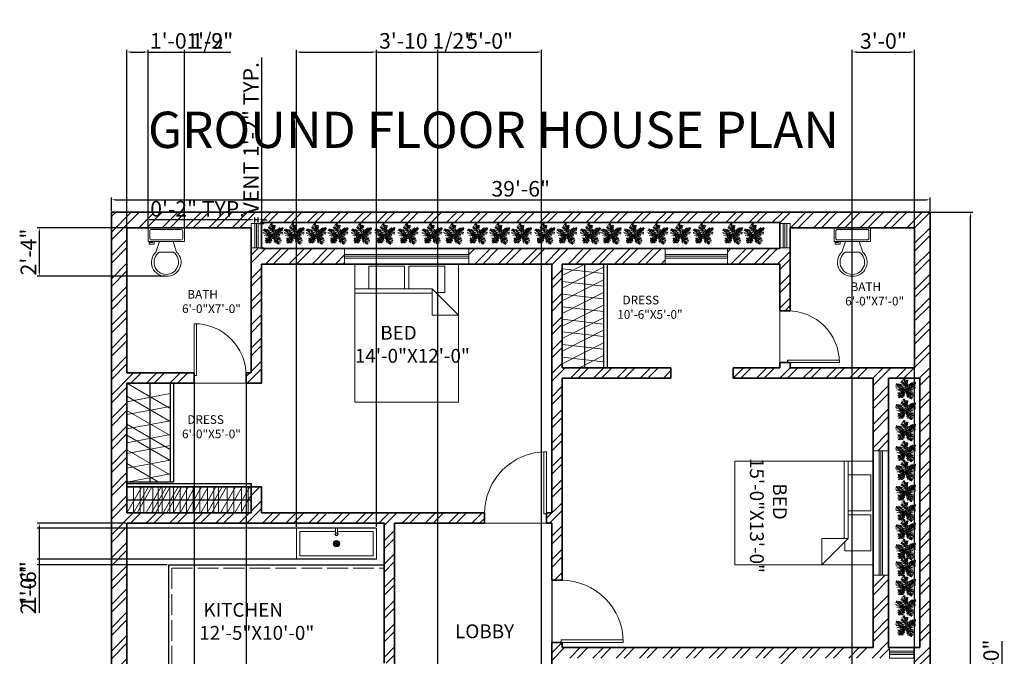
# Model space of a CAD drawing. Units: inches. Extents: x 177 to 1423, y 532 to 2503.
# Tile 4 of 5: x 197 to 768, y 1096 to 1465. Entities that reach past the tile are written whole.
import ezdxf

# ---------------------------------------------------------------- set-up
doc = ezdxf.new("R2010")
doc.units = ezdxf.units.IN
doc.linetypes.add('ACAD_ISO02W100', pattern=[15, 12, -3])
for name, color, linetype, lineweight in [('A-ANNO-DIMS', 2, 'Continuous', 18), ('A-ANNO-TITL', 7, 'Continuous', 35), ('A-AREA-IDEN', 7, 'Continuous', 18), ('A-DOOR', 4, 'Continuous', 18), ('A-FLOR-CASE', 8, 'Continuous', 25), ('A-FLOR-CASE-HIDN', 8, 'ACAD_ISO02W100', 13), ('A-FLOR-CASE-PATT', 252, 'Continuous', 13), ('A-FLOR-FIXT', 9, 'Continuous', 18), ('A-FURN', 8, 'Continuous', 18), ('A-GLAZ', 244, 'Continuous', 18), ('A-WALL', 7, 'Continuous', 35), ('A-WALL-PATT', 252, 'Continuous', 13), ('L-PLNT', 94, 'Continuous', 13)]:
    doc.layers.add(name, color=color, linetype=linetype, lineweight=lineweight)
doc.styles.get("Standard").update_dxf_attribs({"font": 'arial.ttf'})
doc.dimstyles.new('ISO-25', dxfattribs={"dimtxt": 9, "dimasz": 2.5, "dimexe": 1.25, "dimexo": 0.625, "dimtad": 1, "dimlunit": 3, "dimtxsty": 'Standard', "dimcen": 2.5, "dimadec": 0, "dimazin": 0, "dimtfac": 1, "dimtmove": 0, "dimatfit": 3, "dimfxl": 1, "dimarcsym": 0})

# ---------------------------------------------------------------- blocks, each defined once
blk = doc.blocks.new('*U2')
for p, q in [((0, 0), (0, -6)), ((40, 0), (40, -6))]:
    blk.add_line(p, q)
blk.add_lwpolyline([(0, 0), (0, 40), (1.75, 40), (1.75, 0)], close=True)
blk.add_arc((0, 0), 40, 0, 90)
blk = doc.blocks.new('*U3')
for p, q in [((0, 0), (0, -6)), ((-40, 0), (-40, -6))]:
    blk.add_line(p, q)
blk.add_lwpolyline([(0, 0), (0, 40), (-1.75, 40), (-1.75, 0)], close=True)
blk.add_arc((0, 0), 40, 90, 180)
blk = doc.blocks.new('Bed - Queen')
for p, q in [((0, -80.00003), (0, 0)), ((0, 0), (59.99999, 0)), ((59.99999, 0), (59.99999, -80.00003)), ((7.99999, -1.2), (28.79998, -1.2)), ((7.99999, -14.4), (7.99999, -1.2)), ((28.79998, -1.2), (28.79998, -14.4)), ((31.19999, -1.2), (51.99999, -1.2)), ((31.19999, -14.4), (31.19999, -1.2)), ((51.99999, -1.2), (51.99999, -16.4)), ((0, -14.4), (44.8, -14.4)), ((44.8, -16.8), (0, -16.8)), ((59.99999, -29.6), (44.8, -14.4)), ((44.8, -14.4), (44.8, -29.6)), ((51.99999, -16.4), (46.79936, -16.4)), ((44.8, -29.6), (59.99999, -29.6)), ((59.99999, -80.00003), (0, -80.00003))]:
    blk.add_line(p, q)
blk = doc.blocks.new('*U12')
for p, q in [((9.5, -6), (9.5, -2)), ((-10, -8.5), (-8, -8.5)), ((-10, -9.5), (-10, -8.5)), ((-7, -9.5), (-10, -9.5)), ((-8, -8.5), (-8, -8)), ((-7, -8), (-7, -9.5)), ((-4, -8), (-6, -14)), ((4, -8), (6, -14)), ((4, -14), (-4, -14))]:
    blk.add_line(p, q)
blk.add_lwpolyline([(10.5, -8), (10.5, 0), (-10.5, 0), (-10.5, -8)], close=True)
for points in [[(-9.5, -2), (-9.5, -6)], [(8.5, -1), (-8.5, -1)], [(-8.5, -7), (8.5, -7)]]:
    blk.add_lwpolyline(points)
for centre, radius, start, end in [((-8.625, -1.875), 0.8839, 81.8699, 188.1301), ((8.625, -1.875), 0.8839, 351.8699, 98.1301), ((-8.625, -6.125), 0.8839, 171.869898, 278.1301), ((8.625, -6.125), 0.8839, 261.8699, 8.1301), ((-0.4772, -19.9188), 8.0953, 133.01722, 273.38), ((0.0374, -19.8731), 7.127, 124.50543, 269.7), ((-0.0373, -19.8731), 7.127, 270.3, 55.4946), ((0.4773, -19.9188), 8.0953, 266.62, 46.9828)]:
    blk.add_arc(centre, radius, start, end)
blk = doc.blocks.new('*U9')
for p, q in [((9.5, -6), (9.5, -2)), ((-10, -8.5), (-8, -8.5)), ((-10, -9.5), (-10, -8.5)), ((-7, -9.5), (-10, -9.5)), ((-8, -8.5), (-8, -8)), ((-7, -8), (-7, -9.5)), ((-4, -8), (-6, -14)), ((4, -8), (6, -14)), ((4, -14), (-4, -14))]:
    blk.add_line(p, q)
blk.add_lwpolyline([(10.5, -8), (10.5, 0), (-10.5, 0), (-10.5, -8)], close=True)
for points in [[(-9.5, -2), (-9.5, -6)], [(8.5, -1), (-8.5, -1)], [(-8.5, -7), (8.5, -7)]]:
    blk.add_lwpolyline(points)
for centre, radius, start, end in [((-8.625, -1.875), 0.8839, 81.8699, 188.1301), ((8.625, -1.875), 0.8839, 351.8699, 98.1301), ((-8.625, -6.125), 0.8839, 171.869898, 278.1301), ((8.625, -6.125), 0.8839, 261.8699, 8.1301), ((-0.4772, -19.9188), 8.0953, 133.01722, 273.38), ((0.0374, -19.8731), 7.127, 124.50543, 269.7), ((-0.0373, -19.8731), 7.127, 270.3, 55.4946), ((0.4773, -19.9188), 8.0953, 266.62, 46.9828)]:
    blk.add_arc(centre, radius, start, end)
blk = doc.blocks.new('*U11')
for p, q in [((-8.737, 47.138), (-17.069, 52.711)), ((-10.186, 53.64), (-13.084, 55.962)), ((0, 0), (-10.5, 57)), ((-9.099, 51.782), (-6.563, 55.962)), ((-47.498, 19.737), (-55.83, 18.344)), ((-40.615, 13.7), (-55.105, 10.913)), ((-31.5, 4.5), (-52.5, 25.5)), ((-33.37, 6.269), (-52.207, 5.34)), ((-48.585, 21.131), (-49.309, 29.026)), ((-28.299, 3.483), (-47.86, -5.805)), ((-43.513, 28.561), (-42.427, 15.558)), ((-38.442, 26.239), (-34.819, 7.663)), ((-21.416, 3.018), (-38.079, -8.128)), ((-35.544, 28.097), (-24.314, 3.947)), ((0, 0), (-31.5, 4.5)), ((-14.533, 2.09), (-30.834, 25.31)), ((-15.982, 2.09), (-30.11, -9.521)), ((-3.665, 19.273), (-27.574, 35.527)), ((-5.114, 28.097), (-24.676, 40.636)), ((-24.314, 23.917), (-2.941, 13.7)), ((0, 0), (-22.5, -19.5)), ((-7.288, 39.707), (-21.778, 46.673)), ((-6.563, 1.161), (-21.416, -8.128)), ((-20.691, 13.7), (-1.129, 4.876)), ((-7.65, 43.423), (-2.578, 49.46)), ((-5.839, 35.992), (4.667, 48.067)), ((-5.114, 27.632), (10.463, 46.673)), ((-2.941, 16.486), (8.652, 37.85)), ((-1.129, 6.734), (9.014, 26.704)), ((0, 0), (27, 9)), ((0, 0), (18, -22.5)), ((3.942, 1.625), (11.187, 24.381)), ((6.478, 1.625), (26.04, -8.592)), ((10.101, 3.483), (17.708, 26.239)), ((11.187, 3.483), (30.749, -5.805)), ((16.259, 5.805), (23.142, 31.348)), ((18.07, 5.805), (35.096, -3.483)), ((22.055, 7.198), (27.489, 32.277)), ((24.229, 7.663), (46.688, 1.625)), ((27, 9), (48, 36)), ((27.127, 9.056), (31.112, 35.992)), ((29.662, 12.307), (48.137, 6.269)), ((31.836, 30.883), (32.561, 16.486)), ((33.285, 16.486), (48.862, 10.913)), ((35.096, 32.741), (37.27, 22.524)), ((36.183, 19.737), (48.137, 17.88)), ((38.719, 34.134), (41.979, 28.561)), ((40.53, 25.775), (48.862, 24.846)), ((43.791, 29.954), (51.036, 30.883)), ((44.153, 36.456), (45.239, 32.741)), ((-17.431, -15.094), (-42.789, -18.809)), ((-28.299, -29.026), (-42.789, -31.348)), ((-24.314, -21.596), (-42.427, -22.06)), ((-30.834, -34.135), (-42.427, -35.528)), ((-34.457, -39.708), (-40.978, -42.494)), ((-26.849, -26.24), (-40.253, -25.775)), ((-22.5, -19.5), (-37.5, -45)), ((-32.646, -36.921), (-31.921, -44.352)), ((-15.257, -12.772), (-30.11, -12.772)), ((-29.023, -30.884), (-27.936, -43.887)), ((-25.038, -23.918), (-22.865, -45.281)), ((-20.691, -18.345), (-17.793, -44.352)), ((-6.563, -5.805), (-19.967, -9.985)), ((-17.069, -15.094), (-12.721, -40.172)), ((-13.446, -11.378), (-8.737, -32.741)), ((-9.461, -8.592), (-6.201, -23.453)), ((-4.752, -3.483), (-3.665, -14.629)), ((2.493, -3.019), (-1.491, -20.202)), ((1.769, -2.555), (24.229, -9.521)), ((5.029, -6.27), (2.131, -25.775)), ((9.014, -11.378), (3.58, -35.992)), ((14.085, -16.951), (6.478, -40.172)), ((7.565, -9.056), (32.198, -14.629)), ((18.07, -22.524), (8.289, -45.745)), ((12.274, -15.094), (36.907, -18.809)), ((20.244, -30.419), (15.897, -44.816)), ((16.259, -19.738), (36.183, -22.989)), ((18, -22.5), (27, -52.5)), ((18.433, -22.524), (40.53, -29.026)), ((19.157, -25.311), (38.719, -33.206)), ((22.78, -37.85), (19.519, -48.532)), ((21.331, -32.741), (39.081, -40.636)), ((22.78, -38.314), (34.372, -44.816)), ((24.591, -45.745), (23.142, -50.854)), ((24.591, -43.423), (30.749, -47.603)), ((26.764, -49.925), (28.213, -50.854))]:
    blk.add_line(p, q)
blk = doc.blocks.new('*D15')
at = {"layer": 'A-ANNO-DIMS', "color": 0, "lineweight": -2, "transparency": 16777216}
for p, q in [((250.55, 1353.78), (250.55, 1361.61)), ((253.05, 1360.36), (722.05, 1360.36)), ((724.55, 1353.78), (724.55, 1361.61))]:
    blk.add_line(p, q, dxfattribs=at)
at = {"layer": 'A-ANNO-DIMS', "color": 0, "transparency": 16777216}
for points in [[(253.05, 1360.77), (253.05, 1359.94), (250.55, 1360.36)], [(722.05, 1360.77), (722.05, 1359.94), (724.55, 1360.36)]]:
    blk.add_solid(points, dxfattribs=at)
at = {"layer": 'Defpoints', "color": 0, "transparency": 16777216}
for p in [(724.55, 1360.36), (250.55, 1353.15), (724.55, 1353.15)]:
    blk.add_point(p, dxfattribs=at)
at = {"layer": 'A-ANNO-DIMS', "color": 0, "transparency": 16777216, "insert": (487.55, 1365.58), "char_height": 9, "attachment_point": 5}
blk.add_mtext('39\'-6"', dxfattribs=at)
blk = doc.blocks.new('*D16')
at = {"layer": 'A-ANNO-DIMS', "color": 0, "lineweight": -2, "transparency": 16777216}
for p, q in [((725.18, 1353.15), (749.29, 1353.15)), ((748.04, 638.65), (748.04, 1350.65)), ((725.18, 636.15), (749.29, 636.15))]:
    blk.add_line(p, q, dxfattribs=at)
at = {"layer": 'A-ANNO-DIMS', "color": 0, "transparency": 16777216}
for points in [[(747.63, 1350.65), (748.46, 1350.65), (748.04, 1353.15)], [(747.63, 638.65), (748.46, 638.65), (748.04, 636.15)]]:
    blk.add_solid(points, dxfattribs=at)
at = {"layer": 'Defpoints', "color": 0, "transparency": 16777216}
for p in [(724.55, 1353.15), (748.04, 1353.15), (724.55, 636.15)]:
    blk.add_point(p, dxfattribs=at)
at = {"layer": 'A-ANNO-DIMS', "color": 0, "transparency": 16777216, "insert": (742.82, 994.65), "char_height": 9, "attachment_point": 5, "rotation": 90}
blk.add_mtext('59\'-9"', dxfattribs=at)
blk = doc.blocks.new('WIN-GLAZING-72IN')
for p, q in [((72, 2), (0, 2)), ((72, 1), (0, 1)), ((72, 0), (0, 0))]:
    blk.add_line(p, q)
blk = doc.blocks.new('VENT-GLAZING-SHORT')
for p, q in [((14.07, 2), (0, 2)), ((14.07, 1), (0, 1)), ((14.07, 0), (0, 0))]:
    blk.add_line(p, q)
blk = doc.blocks.new('*D26')
at = {"layer": 'A-ANNO-DIMS', "color": 0, "lineweight": -2, "transparency": 16777216}
for p, q in [((337.66, 1346.69), (337.66, 1442.79)), ((336.18, 1346.69), (338.91, 1346.69)), ((337.66, 1335.12), (337.66, 1344.19)), ((336.18, 1332.62), (338.91, 1332.62))]:
    blk.add_line(p, q, dxfattribs=at)
at = {"layer": 'A-ANNO-DIMS', "color": 0, "transparency": 16777216}
for points in [[(337.25, 1344.19), (338.08, 1344.19), (337.66, 1346.69)], [(337.25, 1335.12), (338.08, 1335.12), (337.66, 1332.62)]]:
    blk.add_solid(points, dxfattribs=at)
at = {"layer": 'Defpoints', "color": 0, "transparency": 16777216}
for p in [(335.55, 1346.69), (337.66, 1346.69), (335.55, 1332.62)]:
    blk.add_point(p, dxfattribs=at)
at = {"layer": 'A-ANNO-DIMS', "color": 0, "transparency": 16777216, "insert": (332.52, 1395.99), "char_height": 9, "attachment_point": 5, "rotation": 90}
blk.add_mtext('VENT 1\'-2" TYP.', dxfattribs=at)
blk = doc.blocks.new('*D27')
at = {"layer": 'A-ANNO-DIMS', "color": 0, "lineweight": -2, "transparency": 16777216}
for p, q in [((331.05, 1348.8), (272.44, 1348.8)), ((333.55, 1347.32), (333.55, 1350.05)), ((335.55, 1348.8), (333.55, 1348.8)), ((335.55, 1347.32), (335.55, 1350.05)), ((338.05, 1348.8), (340.55, 1348.8))]:
    blk.add_line(p, q, dxfattribs=at)
at = {"layer": 'A-ANNO-DIMS', "color": 0, "transparency": 16777216}
for points in [[(331.05, 1349.22), (331.05, 1348.39), (333.55, 1348.8)], [(338.05, 1349.22), (338.05, 1348.39), (335.55, 1348.8)]]:
    blk.add_solid(points, dxfattribs=at)
at = {"layer": 'Defpoints', "color": 0, "transparency": 16777216}
for p in [(333.55, 1348.8), (333.55, 1346.69), (335.55, 1346.69)]:
    blk.add_point(p, dxfattribs=at)
at = {"layer": 'A-ANNO-DIMS', "color": 0, "transparency": 16777216, "insert": (300.5, 1354.02), "char_height": 9, "attachment_point": 5}
blk.add_mtext('0\'-2" TYP.', dxfattribs=at)
blk = doc.blocks.new('*D38')
at = {"layer": 'A-ANNO-DIMS', "color": 0, "lineweight": -2, "transparency": 16777216}
for p, q in [((679.55, 810.78), (679.55, 1447.15)), ((682.05, 1445.9), (713.05, 1445.9)), ((715.55, 810.78), (715.55, 1447.15))]:
    blk.add_line(p, q, dxfattribs=at)
at = {"layer": 'A-ANNO-DIMS', "color": 0, "transparency": 16777216}
for points in [[(682.05, 1446.32), (682.05, 1445.49), (679.55, 1445.9)], [(713.05, 1446.32), (713.05, 1445.49), (715.55, 1445.9)]]:
    blk.add_solid(points, dxfattribs=at)
at = {"layer": 'Defpoints', "color": 0, "transparency": 16777216}
for p in [(715.55, 1445.9), (679.55, 810.15), (715.55, 810.15)]:
    blk.add_point(p, dxfattribs=at)
at = {"layer": 'A-ANNO-DIMS', "color": 0, "transparency": 16777216, "insert": (697.55, 1451.13), "char_height": 9, "attachment_point": 5}
blk.add_mtext('3\'-0"', dxfattribs=at)
blk = doc.blocks.new('*D40')
at = {"layer": 'A-ANNO-DIMS', "color": 0, "lineweight": -2, "transparency": 16777216}
for p, q in [((414.55, 1172.53), (414.55, 538.84)), ((505.55, 1172.53), (505.55, 538.84)), ((417.05, 540.09), (503.05, 540.09))]:
    blk.add_line(p, q, dxfattribs=at)
at = {"layer": 'A-ANNO-DIMS', "color": 0, "transparency": 16777216}
for points in [[(417.05, 540.51), (417.05, 539.68), (414.55, 540.09)], [(503.05, 540.51), (503.05, 539.68), (505.55, 540.09)]]:
    blk.add_solid(points, dxfattribs=at)
at = {"layer": 'Defpoints', "color": 0, "transparency": 16777216}
for p in [(414.55, 1173.15), (505.55, 1173.15), (505.55, 540.09)]:
    blk.add_point(p, dxfattribs=at)
at = {"layer": 'A-ANNO-DIMS', "color": 0, "transparency": 16777216, "insert": (460.05, 545.22), "char_height": 9, "attachment_point": 5}
blk.add_mtext('7\'-7"', dxfattribs=at)
blk = doc.blocks.new('*D41')
at = {"layer": 'A-ANNO-DIMS', "color": 0, "lineweight": -2, "transparency": 16777216}
for p, q in [((439.55, 861.78), (439.55, 1447.15)), ((442.05, 1445.9), (497.05, 1445.9)), ((499.55, 861.78), (499.55, 1447.15))]:
    blk.add_line(p, q, dxfattribs=at)
at = {"layer": 'A-ANNO-DIMS', "color": 0, "transparency": 16777216}
for points in [[(442.05, 1446.32), (442.05, 1445.49), (439.55, 1445.9)], [(497.05, 1446.32), (497.05, 1445.49), (499.55, 1445.9)]]:
    blk.add_solid(points, dxfattribs=at)
at = {"layer": 'Defpoints', "color": 0, "transparency": 16777216}
for p in [(499.55, 1445.9), (439.55, 861.15), (499.55, 861.15)]:
    blk.add_point(p, dxfattribs=at)
at = {"layer": 'A-ANNO-DIMS', "color": 0, "transparency": 16777216, "insert": (469.55, 1451.12), "char_height": 9, "attachment_point": 5}
blk.add_mtext('5\'-0"', dxfattribs=at)
blk = doc.blocks.new('*D47')
at = {"layer": 'A-ANNO-DIMS', "color": 0, "lineweight": -2, "transparency": 16777216}
for p, q in [((258.93, 1173.15), (207.55, 1173.15)), ((208.8, 1170.65), (208.8, 1151.65)), ((282.93, 1149.15), (207.55, 1149.15)), ((208.8, 1149.15), (208.8, 1121.33))]:
    blk.add_line(p, q, dxfattribs=at)
at = {"layer": 'A-ANNO-DIMS', "color": 0, "transparency": 16777216}
for points in [[(208.38, 1170.65), (209.22, 1170.65), (208.8, 1173.15)], [(208.38, 1151.65), (209.22, 1151.65), (208.8, 1149.15)]]:
    blk.add_solid(points, dxfattribs=at)
at = {"layer": 'Defpoints', "color": 0, "transparency": 16777216}
for p in [(259.55, 1173.15), (208.8, 1149.15), (283.55, 1149.15)]:
    blk.add_point(p, dxfattribs=at)
at = {"layer": 'A-ANNO-DIMS', "color": 0, "transparency": 16777216, "insert": (203.58, 1133.99), "char_height": 9, "attachment_point": 5, "rotation": 90}
blk.add_mtext('2\'-0"', dxfattribs=at)
blk = doc.blocks.new('*D48')
at = {"layer": 'A-ANNO-DIMS', "color": 0, "lineweight": -2, "transparency": 16777216}
for p, q in [((766.3, 1077.15), (766.3, 1104.98)), ((338.12, 1077.15), (767.55, 1077.15)), ((766.3, 1055.65), (766.3, 1074.65)), ((338.12, 1053.15), (767.55, 1053.15))]:
    blk.add_line(p, q, dxfattribs=at)
at = {"layer": 'A-ANNO-DIMS', "color": 0, "transparency": 16777216}
for points in [[(765.88, 1074.65), (766.72, 1074.65), (766.3, 1077.15)], [(765.88, 1055.65), (766.72, 1055.65), (766.3, 1053.15)]]:
    blk.add_solid(points, dxfattribs=at)
at = {"layer": 'Defpoints', "color": 0, "transparency": 16777216}
for p in [(337.49, 1077.15), (766.3, 1077.15), (337.49, 1053.15)]:
    blk.add_point(p, dxfattribs=at)
at = {"layer": 'A-ANNO-DIMS', "color": 0, "transparency": 16777216, "insert": (761.08, 1092.32), "char_height": 9, "attachment_point": 5, "rotation": 90}
blk.add_mtext('2\'-0"', dxfattribs=at)
blk = doc.blocks.new('*D50')
at = {"layer": 'A-ANNO-DIMS', "color": 0, "lineweight": -2, "transparency": 16777216}
for p, q in [((357.68, 1171.02), (357.68, 1447.15)), ((360.18, 1445.9), (401.53, 1445.9)), ((404.03, 1171.02), (404.03, 1447.15)), ((404.03, 1445.9), (459.66, 1445.9))]:
    blk.add_line(p, q, dxfattribs=at)
at = {"layer": 'A-ANNO-DIMS', "color": 0, "transparency": 16777216}
for points in [[(360.18, 1446.32), (360.18, 1445.49), (357.68, 1445.9)], [(401.53, 1446.32), (401.53, 1445.49), (404.03, 1445.9)]]:
    blk.add_solid(points, dxfattribs=at)
at = {"layer": 'Defpoints', "color": 0, "transparency": 16777216}
for p in [(404.03, 1445.9), (357.68, 1170.39), (404.03, 1170.39)]:
    blk.add_point(p, dxfattribs=at)
at = {"layer": 'A-ANNO-DIMS', "color": 0, "transparency": 16777216, "insert": (433.1, 1451.19), "char_height": 9, "attachment_point": 5}
blk.add_mtext('3\'-10 1/2"', dxfattribs=at)
blk = doc.blocks.new('*D51')
at = {"layer": 'A-ANNO-DIMS', "color": 0, "lineweight": -2, "transparency": 16777216}
for p, q in [((403.41, 1170.39), (207.55, 1170.39)), ((208.8, 1167.89), (208.8, 1154.79)), ((403.41, 1152.29), (207.55, 1152.29)), ((208.8, 1152.29), (208.8, 1125.46))]:
    blk.add_line(p, q, dxfattribs=at)
at = {"layer": 'A-ANNO-DIMS', "color": 0, "transparency": 16777216}
for points in [[(208.38, 1167.89), (209.22, 1167.89), (208.8, 1170.39)], [(208.38, 1154.79), (209.22, 1154.79), (208.8, 1152.29)]]:
    blk.add_solid(points, dxfattribs=at)
at = {"layer": 'Defpoints', "color": 0, "transparency": 16777216}
for p in [(404.03, 1170.39), (208.8, 1152.29), (404.03, 1152.29)]:
    blk.add_point(p, dxfattribs=at)
at = {"layer": 'A-ANNO-DIMS', "color": 0, "transparency": 16777216, "insert": (203.58, 1137.63), "char_height": 9, "attachment_point": 5, "rotation": 90}
blk.add_mtext('1\'-6"', dxfattribs=at)
blk = doc.blocks.new('*D53')
at = {"layer": 'A-ANNO-DIMS', "color": 0, "lineweight": -2, "transparency": 16777216}
for p, q in [((271.82, 1344.78), (271.82, 1447.15)), ((274.32, 1445.9), (290.32, 1445.9)), ((292.82, 1344.78), (292.82, 1447.15)), ((292.82, 1445.9), (319.65, 1445.9))]:
    blk.add_line(p, q, dxfattribs=at)
at = {"layer": 'A-ANNO-DIMS', "color": 0, "transparency": 16777216}
for points in [[(274.32, 1446.32), (274.32, 1445.49), (271.82, 1445.9)], [(290.32, 1446.32), (290.32, 1445.49), (292.82, 1445.9)]]:
    blk.add_solid(points, dxfattribs=at)
at = {"layer": 'Defpoints', "color": 0, "transparency": 16777216}
for p in [(292.82, 1445.9), (271.82, 1344.15), (292.82, 1344.15)]:
    blk.add_point(p, dxfattribs=at)
at = {"layer": 'A-ANNO-DIMS', "color": 0, "transparency": 16777216, "insert": (307.49, 1451.12), "char_height": 9, "attachment_point": 5}
blk.add_mtext('1\'-9"', dxfattribs=at)
blk = doc.blocks.new('*D54')
at = {"layer": 'A-ANNO-DIMS', "color": 0, "lineweight": -2, "transparency": 16777216}
for p, q in [((271.2, 1344.15), (207.55, 1344.15)), ((208.8, 1341.65), (208.8, 1318.65)), ((281.7, 1316.15), (207.55, 1316.15))]:
    blk.add_line(p, q, dxfattribs=at)
at = {"layer": 'A-ANNO-DIMS', "color": 0, "transparency": 16777216}
for points in [[(208.38, 1341.65), (209.22, 1341.65), (208.8, 1344.15)], [(208.38, 1318.65), (209.22, 1318.65), (208.8, 1316.15)]]:
    blk.add_solid(points, dxfattribs=at)
at = {"layer": 'Defpoints', "color": 0, "transparency": 16777216}
for p in [(271.82, 1344.15), (208.8, 1316.15), (282.32, 1316.15)]:
    blk.add_point(p, dxfattribs=at)
at = {"layer": 'A-ANNO-DIMS', "color": 0, "transparency": 16777216, "insert": (203.66, 1330.15), "char_height": 9, "attachment_point": 5, "rotation": 90}
blk.add_mtext('2\'-4"', dxfattribs=at)
blk = doc.blocks.new('*D55')
at = {"layer": 'A-ANNO-DIMS', "color": 0, "lineweight": -2, "transparency": 16777216}
for p, q in [((259.55, 1344.78), (259.55, 1447.15)), ((262.05, 1445.9), (269.32, 1445.9)), ((271.82, 1344.78), (271.82, 1447.15)), ((271.82, 1445.9), (319.62, 1445.9))]:
    blk.add_line(p, q, dxfattribs=at)
at = {"layer": 'A-ANNO-DIMS', "color": 0, "transparency": 16777216}
for points in [[(262.05, 1446.32), (262.05, 1445.49), (259.55, 1445.9)], [(269.32, 1446.32), (269.32, 1445.49), (271.82, 1445.9)]]:
    blk.add_solid(points, dxfattribs=at)
at = {"layer": 'Defpoints', "color": 0, "transparency": 16777216}
for p in [(271.82, 1445.9), (259.55, 1344.15), (271.82, 1344.15)]:
    blk.add_point(p, dxfattribs=at)
at = {"layer": 'A-ANNO-DIMS', "color": 0, "transparency": 16777216, "insert": (296.97, 1451.18), "char_height": 9, "attachment_point": 5}
blk.add_mtext('1\'-0 1/2"', dxfattribs=at)
blk = doc.blocks.new('*D56')
at = {"layer": 'A-ANNO-DIMS', "color": 0, "lineweight": -2, "transparency": 16777216}
for p, q in [((298.55, 1259.53), (298.55, 538.84)), ((328.55, 1259.53), (328.55, 538.84)), ((301.05, 540.09), (326.05, 540.09))]:
    blk.add_line(p, q, dxfattribs=at)
at = {"layer": 'A-ANNO-DIMS', "color": 0, "transparency": 16777216}
for points in [[(301.05, 540.51), (301.05, 539.68), (298.55, 540.09)], [(326.05, 540.51), (326.05, 539.68), (328.55, 540.09)]]:
    blk.add_solid(points, dxfattribs=at)
at = {"layer": 'Defpoints', "color": 0, "transparency": 16777216}
for p in [(298.55, 1260.15), (328.55, 1260.15), (328.55, 540.09)]:
    blk.add_point(p, dxfattribs=at)
at = {"layer": 'A-ANNO-DIMS', "color": 0, "transparency": 16777216, "insert": (313.55, 545.31), "char_height": 9, "attachment_point": 5}
blk.add_mtext('2\'-6"', dxfattribs=at)

msp = doc.modelspace()

# ---------------------------------------------------------------- hatches: boundary and pattern name
at = {"layer": 'A-FLOR-CASE-PATT'}
h = msp.add_hatch(dxfattribs=at)
h.set_pattern_fill('ANSI31', color=256, scale=2.05074, angle=-18.1832, style=0)
h.paths.add_polyline_path([(511.55, 1263.154), (535.55, 1263.154), (535.55, 1323.154), (511.55, 1323.154)])
h = msp.add_hatch(dxfattribs=at)
h.set_pattern_fill('ANSI31', color=256, scale=2.282986, angle=128.4752, style=0)
h.paths.add_polyline_path([(511.55, 1263.154), (535.55, 1263.154), (535.55, 1323.154), (511.55, 1323.154)])
at = {"layer": 'A-WALL-PATT'}
h = msp.add_hatch(dxfattribs=at)
h.set_pattern_fill('ANSI32', color=256)
h.paths.add_polyline_path([(436.55, 810.154), (427.55, 810.154), (427.55, 711.154), (379.55, 711.154), (379.55, 702.154), (436.55, 702.154)])
h.paths.add_polyline_path([(337.55, 963.154), (331.55, 963.154), (331.55, 951.154), (319.738, 951.154), (319.738, 945.154), (331.55, 945.154), (331.55, 861.154), (328.55, 861.154), (328.55, 855.154), (427.55, 855.154), (427.55, 846.154), (436.55, 846.154), (436.55, 852.154), (439.55, 852.154), (439.55, 861.154), (337.55, 861.154)], flags=17)
h.paths.add_polyline_path([(682.55, 1011.154), (643.55, 1011.154), (643.55, 1095.154), (701.063, 1095.154), (701.063, 1101.154), (700.55, 1101.154), (700.55, 1143.154), (691.55, 1143.154), (691.55, 1101.154), (511.55, 1101.154), (511.55, 1104.154), (505.55, 1104.154), (505.55, 1068.154), (511.55, 1068.154), (511.55, 1095.154), (637.55, 1095.154), (637.55, 1011.154), (511.55, 1011.154), (511.55, 1038.154), (505.55, 1038.154), (505.55, 1005.154), (541.55, 1005.154), (541.55, 1002.154), (547.55, 1002.154), (547.55, 1005.154), (682.55, 1005.154)], flags=17)
h.paths.add_polyline_path([(547.55, 966.154), (541.55, 966.154), (541.55, 861.154), (499.55, 861.154), (499.55, 852.154), (595.55, 852.154), (595.55, 861.154), (547.55, 861.154)], flags=17)
h.paths.add_polyline_path([(724.55, 1353.154), (337.55, 1353.154), (250.55, 1353.154), (250.55, 702.154), (307.55, 702.154), (307.55, 711.154), (259.55, 711.154), (259.55, 855.154), (298.55, 855.154), (298.55, 861.154), (259.55, 861.154), (259.55, 945.154), (298.738, 945.154), (298.738, 951.154), (259.55, 951.154), (259.55, 1047.154), (331.55, 1047.154), (331.55, 1035.154), (337.55, 1035.154), (337.55, 1047.154), (414.55, 1047.154), (414.55, 1056.154), (408.55, 1056.154), (408.55, 1053.154), (259.55, 1053.154), (259.55, 1173.154), (408.55, 1173.154), (408.55, 1092.154), (414.55, 1092.154), (414.55, 1173.154), (466.55, 1173.154), (466.55, 1179.154), (337.55, 1179.154), (337.55, 1194.154), (331.55, 1194.154), (331.55, 1179.154), (259.55, 1179.154), (259.55, 1194.154), (259.55, 1254.154), (298.55, 1254.154), (298.55, 1258.654), (298.55, 1260.154), (259.55, 1260.154), (259.55, 1344.154), (331.55, 1344.154), (331.55, 1346.691), (337.55, 1346.691), (337.55, 1347.154), (637.55, 1347.154), (637.55, 1346.676), (643.55, 1346.676), (643.55, 1344.154), (715.55, 1344.154), (715.55, 1263.154), (643.55, 1263.154), (643.55, 1266.154), (642.05, 1266.154), (637.55, 1266.154), (637.55, 1263.154), (610.55, 1263.154), (610.55, 1257.154), (691.55, 1257.154), (691.55, 1215.154), (700.55, 1215.154), (700.55, 1257.154), (718.55, 1257.154), (718.55, 1101.154), (715.137, 1101.154), (715.137, 1095.154), (715.55, 1095.154), (715.55, 1011.154), (712.55, 1011.154), (712.55, 1009.654), (712.55, 1005.154), (715.55, 1005.154), (715.55, 861.154), (667.55, 861.154), (667.55, 852.154), (724.55, 852.154)])
h.paths.add_polyline_path([(571.243, 1332.154), (457.55, 1332.154), (457.55, 1323.154), (505.55, 1323.154), (505.55, 1179.154), (502.55, 1179.154), (502.55, 1178.554), (502.55, 1173.154), (505.55, 1173.154), (505.55, 1140.154), (510.95, 1140.154), (511.55, 1140.154), (511.55, 1257.154), (574.55, 1257.154), (574.55, 1263.154), (511.55, 1263.154), (511.55, 1323.154), (571.243, 1323.154)], flags=17)
h.paths.add_polyline_path([(385.55, 1332.154), (337.55, 1332.154), (337.55, 1332.617), (331.55, 1332.617), (331.55, 1260.154), (328.55, 1260.154), (328.55, 1254.154), (337.55, 1254.154), (337.55, 1323.154), (385.55, 1323.154)], flags=17)
h.paths.add_polyline_path([(643.55, 1332.601), (637.55, 1332.601), (637.55, 1332.154), (607.243, 1332.154), (607.243, 1323.154), (637.55, 1323.154), (637.55, 1296.154), (642.05, 1296.154), (643.55, 1296.154)], flags=17)

# ---------------------------------------------------------------- linework, layer by layer
at = {"layer": 'A-DOOR'}
for p, q in [((637.55, 1296.154), (637.55, 1266.154)), ((298.55, 1254.154), (328.55, 1254.154)), ((502.55, 1173.154), (466.55, 1173.154)), ((505.55, 1104.154), (505.55, 1140.154))]:
    msp.add_line(p, q, dxfattribs=at)
at = {"layer": 'A-FLOR-CASE'}
for p, q in [((524.572, 1323.154), (524.572, 1263.154)), ((535.55, 1323.154), (535.55, 1263.154)), ((537.55, 1323.154), (537.55, 1263.154)), ((273.05, 1197.154), (273.05, 1254.154)), ((284.55, 1254.154), (284.55, 1197.154)), ((286.55, 1254.154), (286.55, 1197.154)), ((259.55, 1197.154), (286.55, 1197.154)), ((259.55, 1196.154), (331.55, 1196.154)), ((259.55, 1186.654), (331.55, 1186.654)), ((283.55, 1149.154), (283.55, 1077.154)), ((283.55, 1149.154), (408.55, 1149.154))]:
    msp.add_line(p, q, dxfattribs=at)
at = {"layer": 'A-FLOR-CASE-HIDN'}
for q in [(408.55, 1147.154), (285.55, 1079.154)]:
    msp.add_line((285.55, 1147.154), q, dxfattribs=at)
at = {"layer": 'A-FLOR-CASE-PATT'}
for p, q in [((259.55, 1254.154), (284.55, 1239.54)), ((259.55, 1243.443), (284.55, 1248.167)), ((259.55, 1246.729), (284.55, 1232.115)), ((259.55, 1236.018), (284.55, 1240.741)), ((259.55, 1238.513), (284.55, 1223.9)), ((259.55, 1227.802), (284.55, 1232.526)), ((259.55, 1230.503), (284.55, 1215.889)), ((259.55, 1219.792), (284.55, 1224.516)), ((259.55, 1224.154), (284.55, 1209.54)), ((259.55, 1213.443), (284.55, 1218.167)), ((259.55, 1215.715), (284.55, 1201.101)), ((259.55, 1205.004), (284.55, 1209.728)), ((259.55, 1207.705), (277.6, 1197.154)), ((259.55, 1196.994), (284.55, 1201.718)), ((259.55, 1179.154), (268.127, 1194.154)), ((263.391, 1194.154), (263.391, 1179.154)), ((263.391, 1179.154), (271.968, 1194.154)), ((265.447, 1179.154), (274.023, 1194.154)), ((267.231, 1194.154), (267.231, 1179.154)), ((269.287, 1194.154), (269.287, 1179.154)), ((270.725, 1179.154), (279.302, 1194.154)), ((273.842, 1179.154), (282.419, 1194.154)), ((274.565, 1194.154), (274.565, 1179.154)), ((276.013, 1179.154), (284.59, 1194.154)), ((277.682, 1194.154), (277.682, 1179.154)), ((279.853, 1194.154), (279.853, 1179.154)), ((280.587, 1179.154), (289.164, 1194.154)), ((282.598, 1179.154), (291.175, 1194.154)), ((284.428, 1194.154), (284.428, 1179.154)), ((286.439, 1194.154), (286.439, 1179.154)), ((286.439, 1179.154), (295.016, 1194.154)), ((290.279, 1194.154), (290.279, 1179.154)), ((290.279, 1179.154), (298.856, 1194.154)), ((294.12, 1194.154), (294.12, 1179.154)), ((294.12, 1179.154), (302.696, 1194.154)), ((297.96, 1194.154), (297.96, 1179.154)), ((297.96, 1179.154), (306.537, 1194.154)), ((301.8, 1194.154), (301.8, 1179.154)), ((302.367, 1179.154), (310.943, 1194.154)), ((306.036, 1179.154), (314.613, 1194.154)), ((306.207, 1194.154), (306.207, 1179.154)), ((308.66, 1179.154), (317.237, 1194.154)), ((309.877, 1194.154), (309.877, 1179.154)), ((312.5, 1194.154), (312.5, 1179.154)), ((313.788, 1179.154), (322.364, 1194.154)), ((317.628, 1194.154), (317.628, 1179.154)), ((317.628, 1179.154), (326.205, 1194.154)), ((321.468, 1194.154), (321.468, 1179.154)), ((322.082, 1179.154), (330.659, 1194.154)), ((325.923, 1194.154), (325.923, 1179.154)), ((329.763, 1194.154), (329.763, 1179.154)), ((325.923, 1179.862), (331.55, 1189.704))]:
    msp.add_line(p, q, dxfattribs=at)
at = {"layer": 'A-FLOR-FIXT'}
for p, q in [((380.256, 1167.478), (380.256, 1170.391)), ((381.456, 1167.478), (381.456, 1170.391)), ((380.856, 1163.204), (380.856, 1159.478)), ((378.993, 1161.341), (382.719, 1161.341)), ((382.144, 1159.995), (379.568, 1162.687)), ((379.641, 1159.928), (382.071, 1162.754))]:
    msp.add_line(p, q, dxfattribs=at)
msp.add_lwpolyline([(357.68, 1170.391), (404.032, 1170.391), (404.032, 1152.29), (357.68, 1152.29)], close=True, dxfattribs=at)
msp.add_lwpolyline([(381.456, 1168.391), (402.032, 1168.391), (402.032, 1154.29), (359.68, 1154.29), (359.68, 1168.391), (380.256, 1168.391)], dxfattribs=at)
for centre, radius in [((380.856, 1161.341), 1.863), ((380.856, 1166.798), 0.907), ((380.856, 1166.798), 0.607), ((380.856, 1161.341), 1.263)]:
    msp.add_circle(centre, radius, dxfattribs=at)
at = {"layer": 'A-GLAZ'}
for p, q in [((571.243, 1328.654), (607.243, 1328.654)), ((571.243, 1327.654), (607.243, 1327.654)), ((571.243, 1326.654), (607.243, 1326.654))]:
    msp.add_line(p, q, dxfattribs=at)
for points in [[(337.55, 1346.691), (337.55, 1332.617), (331.55, 1332.617), (331.55, 1346.691)], [(643.55, 1346.676), (643.55, 1332.601), (637.55, 1332.601), (637.55, 1346.676)], [(385.55, 1332.154), (457.55, 1332.154), (457.55, 1323.154), (385.55, 1323.154)], [(571.243, 1332.154), (607.243, 1332.154), (607.243, 1323.154), (571.243, 1323.154)], [(700.55, 1215.154), (700.55, 1143.154), (691.55, 1143.154), (691.55, 1215.154)], [(701.063, 1101.154), (715.137, 1101.154), (715.137, 1095.154), (701.063, 1095.154)]]:
    msp.add_lwpolyline(points, close=True, dxfattribs=at)
at = {"layer": 'A-WALL'}
for p, q in [((250.55, 1353.154), (250.55, 636.154)), ((250.55, 1353.154), (337.55, 1353.154)), ((337.55, 1353.154), (724.55, 1353.154)), ((724.55, 1353.154), (724.55, 636.154)), ((337.55, 1347.154), (637.55, 1347.154)), ((337.55, 1347.154), (337.55, 1332.154)), ((637.55, 1347.154), (637.55, 1332.154)), ((259.55, 1344.154), (331.55, 1344.154)), ((259.55, 1344.154), (259.55, 1260.154)), ((331.55, 1344.154), (331.55, 1260.154)), ((643.55, 1344.154), (643.55, 1296.154)), ((643.55, 1344.154), (715.55, 1344.154)), ((715.55, 1344.154), (715.55, 1263.154)), ((337.55, 1332.154), (637.55, 1332.154)), ((337.55, 1323.154), (505.55, 1323.154)), ((337.55, 1323.154), (337.55, 1254.154)), ((505.55, 1323.154), (505.55, 1179.154)), ((511.55, 1323.154), (511.55, 1263.154)), ((511.55, 1323.154), (637.55, 1323.154)), ((637.55, 1323.154), (637.55, 1296.154)), ((637.55, 1296.154), (643.55, 1296.154)), ((637.55, 1266.154), (643.55, 1266.154)), ((637.55, 1266.154), (637.55, 1263.154)), ((643.55, 1266.154), (643.55, 1263.154)), ((259.55, 1260.154), (298.55, 1260.154)), ((298.55, 1260.154), (298.55, 1254.154)), ((328.55, 1260.154), (328.55, 1254.154)), ((328.55, 1260.154), (331.55, 1260.154)), ((511.55, 1263.154), (574.55, 1263.154)), ((574.55, 1263.154), (574.55, 1257.154)), ((610.55, 1263.154), (610.55, 1257.154)), ((610.55, 1263.154), (637.55, 1263.154)), ((643.55, 1263.154), (715.55, 1263.154)), ((511.55, 1257.154), (574.55, 1257.154)), ((511.55, 1257.154), (511.55, 1140.154)), ((610.55, 1257.154), (691.55, 1257.154)), ((691.55, 1257.154), (691.55, 1101.154)), ((700.55, 1257.154), (700.55, 1101.154)), ((700.55, 1257.154), (718.55, 1257.154)), ((718.55, 1257.154), (718.55, 1101.154)), ((259.55, 1254.154), (259.55, 1194.154)), ((259.55, 1254.154), (298.55, 1254.154)), ((328.55, 1254.154), (337.55, 1254.154)), ((259.55, 1194.154), (259.55, 1179.154)), ((259.55, 1194.154), (337.55, 1194.154)), ((331.55, 1196.154), (331.55, 1179.154)), ((337.55, 1194.154), (337.55, 1179.154)), ((259.55, 1179.154), (331.55, 1179.154)), ((337.55, 1179.154), (466.55, 1179.154)), ((466.55, 1173.154), (466.55, 1179.154)), ((502.55, 1173.154), (502.55, 1179.154)), ((502.55, 1179.154), (505.55, 1179.154)), ((259.55, 1173.154), (408.55, 1173.154)), ((259.55, 1173.154), (259.55, 1053.154)), ((408.55, 1173.154), (408.55, 1092.154)), ((414.55, 1173.154), (414.55, 1092.154)), ((414.55, 1173.154), (466.55, 1173.154)), ((502.55, 1173.154), (505.55, 1173.154)), ((505.55, 1173.154), (505.55, 1140.154)), ((511.55, 1140.154), (505.55, 1140.154)), ((511.55, 1104.154), (505.55, 1104.154)), ((505.55, 1104.154), (505.55, 1068.154)), ((511.55, 1104.154), (511.55, 1101.154)), ((511.55, 1101.154), (691.55, 1101.154)), ((700.55, 1101.154), (718.55, 1101.154))]:
    msp.add_line(p, q, dxfattribs=at)

# ---------------------------------------------------------------- block references
at = {"layer": 'A-DOOR'}
for name, p, xscale, yscale, zscale, rotation in [('*U3', (642.05, 1266.154), 0.7499999999999976, 0.7499999999999976, 0.7499999999999976, 270.0000000000002), ('*U2', (502.55, 1178.554), -0.9000000000000095, 0.9000000000000095, 0.9000000000000095, 1.5987e-12), ('*U2', (510.95, 1104.154), -0.9000000000000095, 0.9000000000000095, 0.9000000000000095, 270)]:
    msp.add_blockref(name, p, dxfattribs=dict(at, xscale=xscale, yscale=yscale, zscale=zscale, rotation=rotation))
at = {"layer": 'A-DOOR', "xscale": 0.7499999999999976, "yscale": 0.7499999999999976, "zscale": 0.7499999999999976}
msp.add_blockref('*U2', (298.55, 1258.654), dxfattribs=at)
at = {"layer": 'A-FLOR-FIXT'}
for name, p in [('*U12', (282.323, 1344.154)), ('*U9', (679.55, 1344.154))]:
    msp.add_blockref(name, p, dxfattribs=at)
at = {"layer": 'A-FURN'}
msp.add_blockref('Bed - Queen', (391.55, 1323.154), dxfattribs=at)
at = {"layer": 'A-FURN', "rotation": 270}
msp.add_blockref('Bed - Queen', (691.55, 1209.154), dxfattribs=at)
at = {"layer": 'A-GLAZ'}
for name, p, rotation in [('VENT-GLAZING-SHORT', (335.551, 1332.617), 90.00000000000571), ('VENT-GLAZING-SHORT', (641.551, 1332.601), 90.0000000000061), ('WIN-GLAZING-72IN', (457.551, 1328.654), 180), ('WIN-GLAZING-72IN', (695.05, 1215.155), 270.0000000000003), ('VENT-GLAZING-SHORT', (715.137, 1099.154), 180)]:
    msp.add_blockref(name, p, dxfattribs=dict(at, rotation=rotation))
at = {"layer": 'L-PLNT', "xscale": 0.1117025751797268, "yscale": 0.1117025751797268, "zscale": 0.1117025751797268}
for p in [(344.427, 1340.315), (356.698, 1340.315), (369.415, 1340.315), (382.112, 1340.315), (395.61, 1340.315), (409.201, 1340.315), (422.639, 1340.315), (436.536, 1340.315), (449.058, 1340.315), (462.778, 1340.315), (475.63, 1340.315), (488.305, 1340.315), (501.773, 1340.315), (514.601, 1340.315), (528.192, 1340.315), (540.256, 1340.315), (553.427, 1340.315), (567.208, 1340.315), (580.341, 1340.315), (593.474, 1340.315), (610.54, 1340.315), (622.947, 1340.315), (710.712, 1250.793), (710.712, 1238.812), (710.712, 1226.45), (710.712, 1214.484), (710.712, 1203.387), (710.712, 1191.447), (710.712, 1179.896), (710.712, 1169.155), (710.712, 1157.7), (710.712, 1147.762), (710.712, 1136.696), (710.712, 1125.009), (710.712, 1113.361)]:
    msp.add_blockref('*U11', p, dxfattribs=at)

# ---------------------------------------------------------------- texts
at = {"layer": 'A-ANNO-TITL', "insert": (271.73, 1411.359), "char_height": 21, "attachment_point": 1}
msp.add_mtext_dynamic_manual_height_columns('GROUND FLOOR HOUSE PLAN', width=439.21207, gutter_width=12.5, heights=[0], dxfattribs=at)
at = {"layer": 'A-AREA-IDEN', "attachment_point": 1}
for s, width, insert, char_height in [('  BATH\\P6\'-0"X7\'-0"', 31.84746, (675.455, 1312.555), 5), ('  BATH\\P6\'-0"X7\'-0"', 31.84746, (291.455, 1308.168), 5), ('  DRESS\\P10\'-6"X5\'-0"', 35.8781, (543.455, 1304.841), 5), ('      BED\\P14\'-0"X12\'-0"', 64.26677, (391.534, 1287.42), 8), ('  DRESS\\P6\'-0"X5\'-0"', 31.84746, (291.455, 1235.679), 5), (' KITCHEN\\P12\'-5"X10\'-0"', 64.26677, (301.42, 1127.048), 8), ('LOBBY', 35.9173, (449.561, 1114.613), 8)]:
    msp.add_mtext_dynamic_manual_height_columns(s, width=width, gutter_width=12.5, heights=[0], dxfattribs=dict(at, insert=insert, char_height=char_height))
at = {"layer": 'A-AREA-IDEN', "insert": (641.602, 1210.951), "char_height": 8, "attachment_point": 1, "rotation": 270}
msp.add_mtext_dynamic_manual_height_columns('      BED\\P15\'-0"X13\'-0"', width=64.26677, gutter_width=12.5, heights=[0], dxfattribs=at)

# ---------------------------------------------------------------- dimensions: what is measured, and where the dimension line sits
at = {"layer": 'A-ANNO-DIMS'}
for base, p1, p2, override, picture, middle in [((271.823, 1445.904), (259.55, 1344.154), (271.823, 1344.154), {"dimdec": 1, "dimlfac": 1, "dimrnd": 0, "dimzin": 1, "dimdsep": 46, "dimlunit": 4, "dimfrac": 2}, '*D55', (296.972, 1451.183)), ((404.032, 1445.904), (357.68, 1170.391), (404.032, 1170.391), {"dimdec": 1, "dimlfac": 1, "dimrnd": 0, "dimzin": 1, "dimdsep": 46, "dimlunit": 4, "dimfrac": 2}, '*D50', (433.098, 1451.186)), ((292.823, 1445.904), (271.823, 1344.154), (292.823, 1344.154), {"dimdec": 1, "dimlfac": 1, "dimrnd": 0, "dimzin": 1, "dimdsep": 46, "dimlunit": 4, "dimfrac": 2}, '*D53', (307.486, 1451.124)), ((499.55, 1445.904), (439.55, 861.154), (499.55, 861.154), {"dimdec": 1, "dimlfac": 1, "dimrnd": 0, "dimzin": 1, "dimdsep": 46, "dimlunit": 4, "dimfrac": 2}, '*D41', (469.55, 1451.124)), ((715.55, 1445.904), (679.55, 810.154), (715.55, 810.154), {"dimdec": 1, "dimlfac": 1, "dimrnd": 0, "dimzin": 1, "dimdsep": 46, "dimlunit": 4, "dimfrac": 2}, '*D38', (697.55, 1451.127)), ((724.55, 1360.358), (250.55, 1353.154), (724.55, 1353.154), {"dimclrd": 0, "dimclre": 0, "dimclrt": 0}, '*D15', (487.55, 1365.581)), ((328.55, 540.092), (298.55, 1260.154), (328.55, 1260.154), {"dimdec": 1, "dimlfac": 1, "dimrnd": 0, "dimzin": 1, "dimdsep": 46, "dimlunit": 4, "dimfrac": 2}, '*D56', (313.55, 545.313)), ((505.55, 540.092), (414.55, 1173.154), (505.55, 1173.154), {"dimdec": 1, "dimlfac": 1, "dimrnd": 0, "dimzin": 1, "dimdsep": 46, "dimlunit": 4, "dimfrac": 2}, '*D40', (460.05, 545.217))]:
    dim = msp.add_linear_dim(base=base, p1=p1, p2=p2, dimstyle='ISO-25', override=override, dxfattribs=at)
    dim.commit()
    dim.dimension.update_dxf_attribs({"geometry": picture, "text_midpoint": middle})
for base, p1, p2, angle, text, picture, middle in [((337.662, 1346.691), (335.55, 1332.617), (335.55, 1346.691), 90, 'VENT <> TYP.', '*D26', (332.515, 1395.992)), ((333.55, 1348.803), (335.55, 1346.691), (333.55, 1346.691), 180, '<> TYP.', '*D27', (300.496, 1354.023))]:
    dim = msp.add_linear_dim(base=base, p1=p1, p2=p2, angle=angle, text=text, dimstyle='ISO-25', override={"dimdec": 1, "dimlfac": 1, "dimrnd": 0, "dimzin": 1, "dimdsep": 46, "dimlunit": 4, "dimfrac": 2}, dxfattribs=at)
    dim.commit()
    dim.dimension.update_dxf_attribs({"geometry": picture, "text_midpoint": middle})
for base, p1, p2, override, picture, middle in [((748.044, 1353.154), (724.55, 636.154), (724.55, 1353.154), {"dimclrd": 0, "dimclre": 0, "dimclrt": 0}, '*D16', (742.824, 994.654)), ((208.8, 1316.154), (271.823, 1344.154), (282.323, 1316.154), {"dimdec": 1, "dimlfac": 1, "dimrnd": 0, "dimzin": 1, "dimdsep": 46, "dimlunit": 4, "dimfrac": 2}, '*D54', (203.657, 1330.154)), ((208.8, 1149.154), (259.55, 1173.154), (283.55, 1149.154), {"dimdec": 1, "dimlfac": 1, "dimrnd": 0, "dimzin": 1, "dimdsep": 46, "dimlunit": 4, "dimfrac": 2}, '*D47', (203.58, 1133.99)), ((208.8, 1152.29), (404.032, 1170.391), (404.032, 1152.29), {"dimdec": 1, "dimlfac": 1, "dimrnd": 0, "dimzin": 1, "dimdsep": 46, "dimlunit": 4, "dimfrac": 2}, '*D51', (203.58, 1137.627)), ((766.3, 1077.154), (337.493, 1053.154), (337.493, 1077.154), {"dimdec": 1, "dimlfac": 1, "dimrnd": 0, "dimzin": 1, "dimdsep": 46, "dimlunit": 4, "dimfrac": 2}, '*D48', (761.08, 1092.318))]:
    dim = msp.add_linear_dim(base=base, p1=p1, p2=p2, angle=90, dimstyle='ISO-25', override=override, dxfattribs=at)
    dim.commit()
    dim.dimension.update_dxf_attribs({"geometry": picture, "text_midpoint": middle})

doc.saveas('drawing.dxf')
